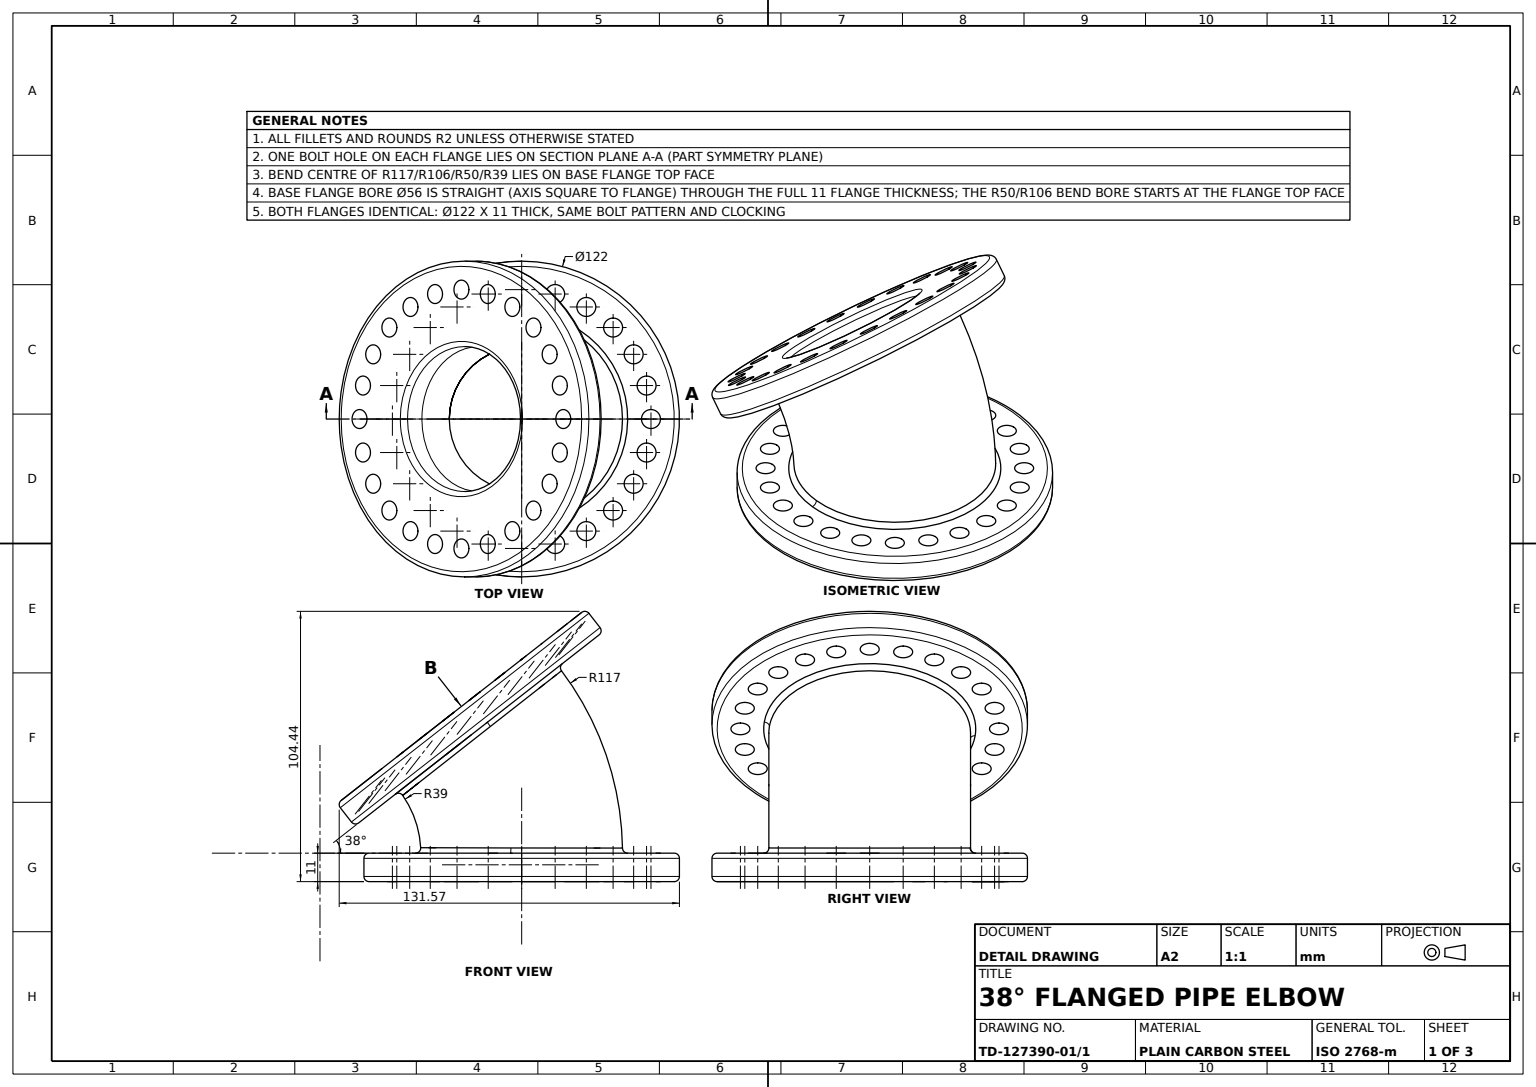
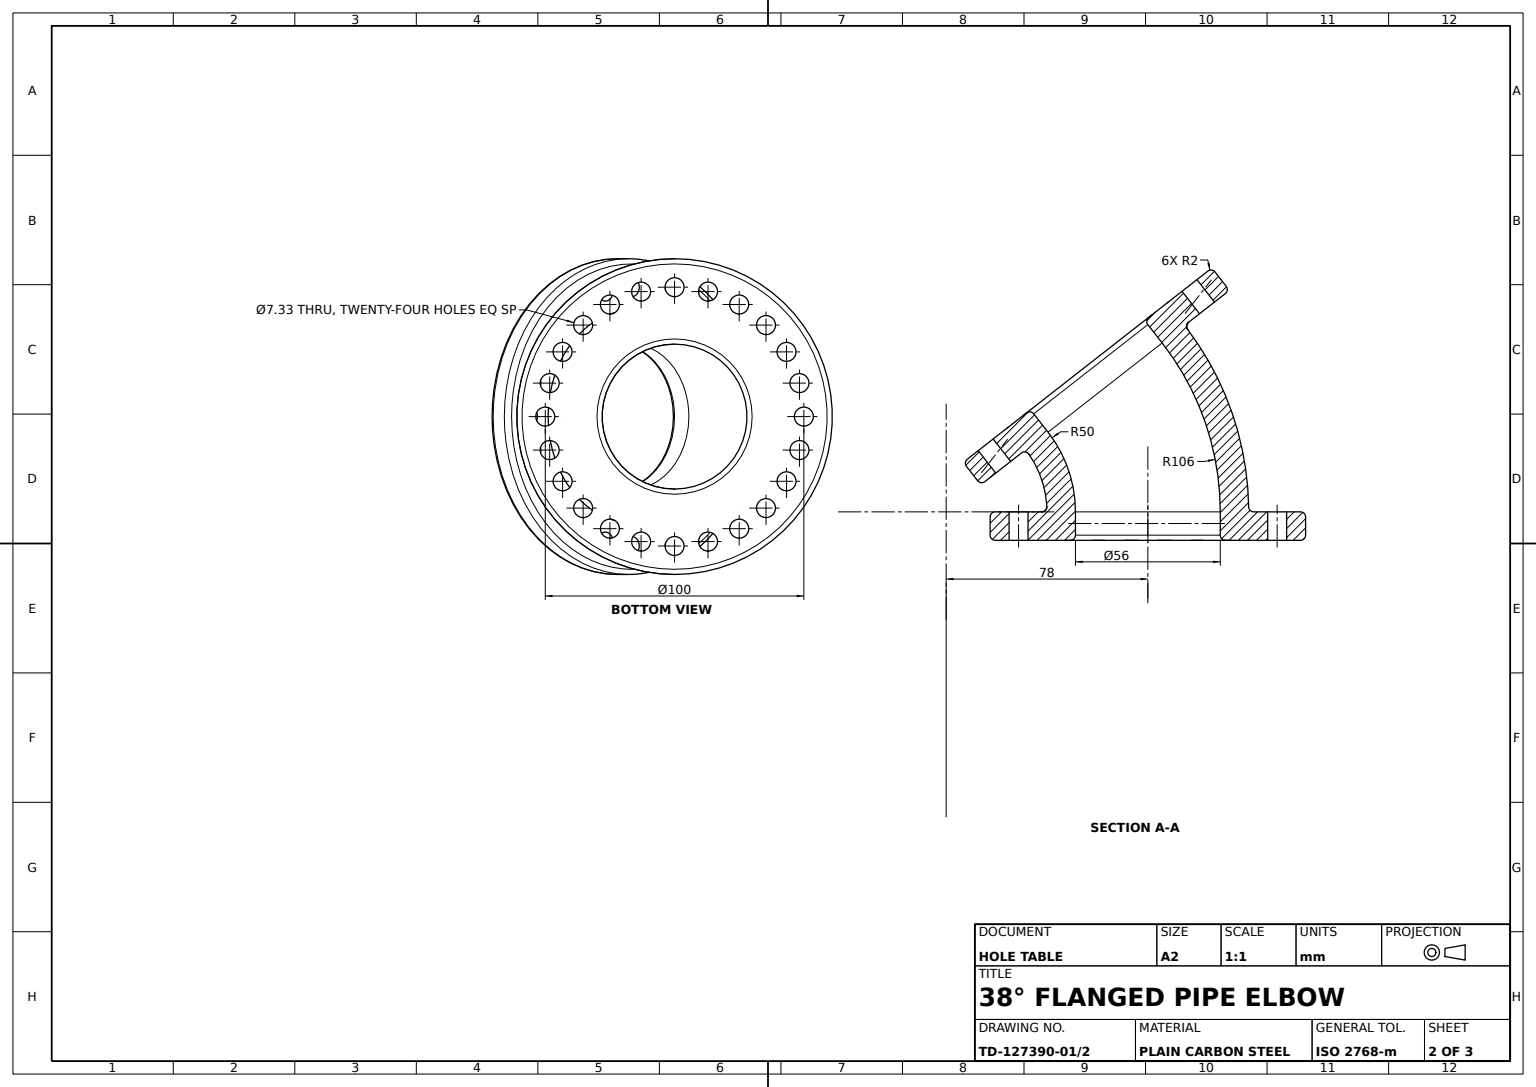
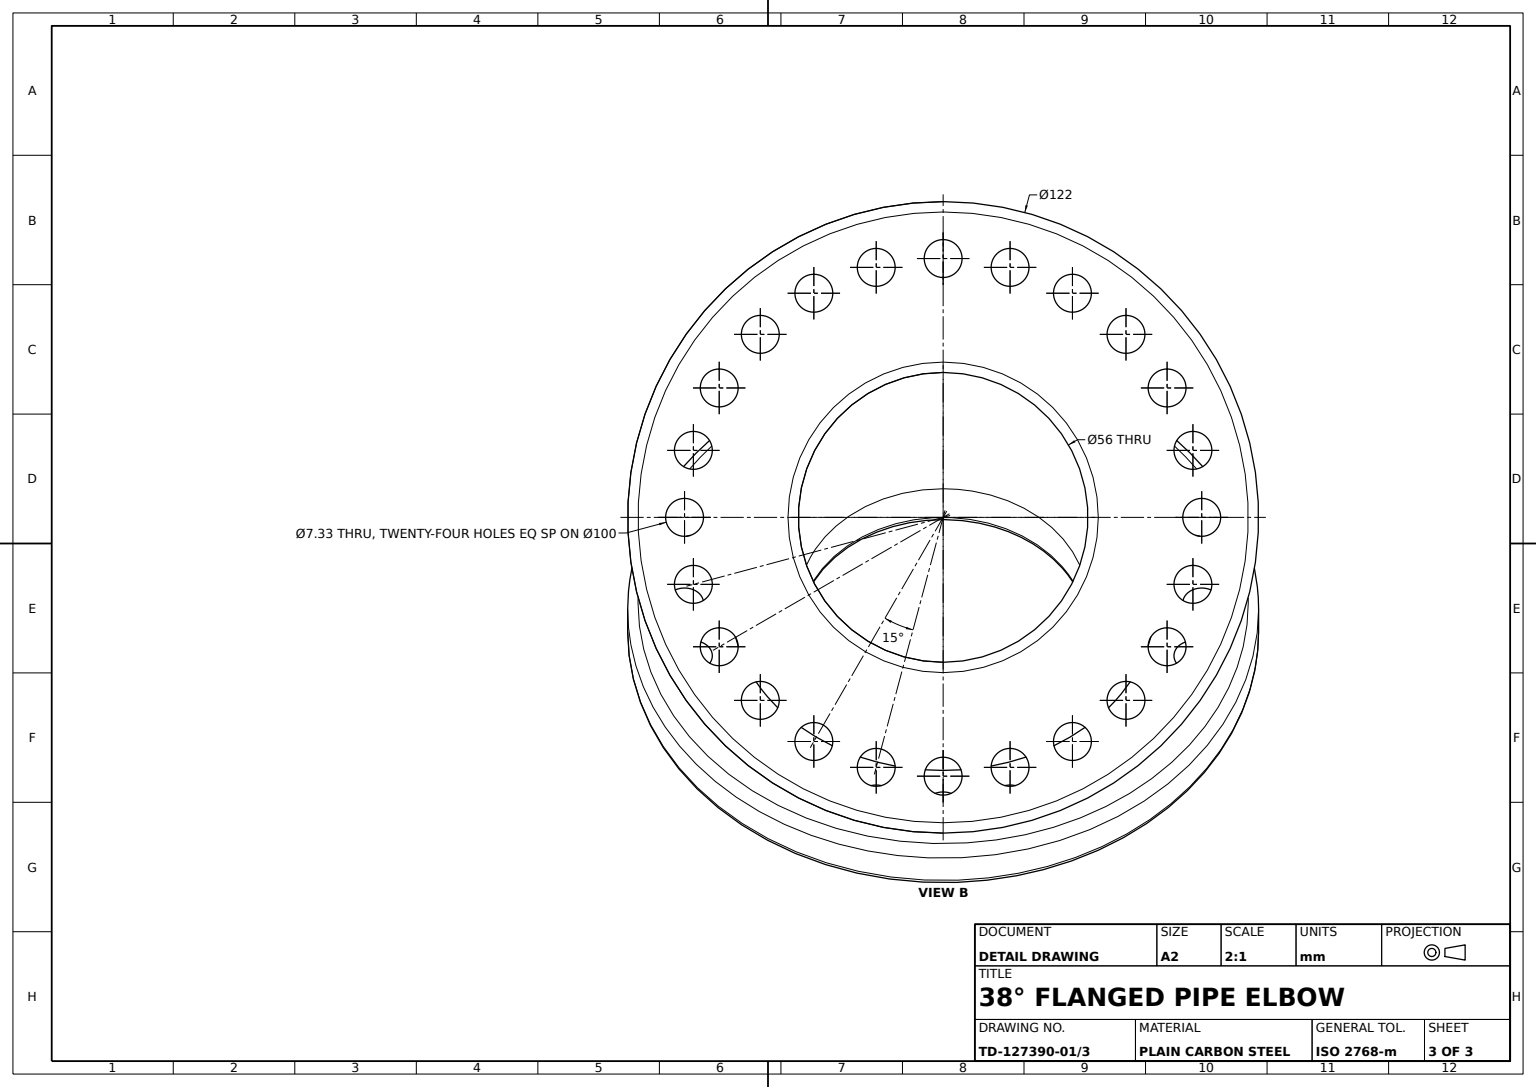
from build123d import *

# Parameters (mm, degrees)
BASE_FLANGE_SKETCH_R       = 61
BASE_FLANGE_SKETCH_R_2     = 28
BASE_FLANGE_SKETCH_R_3     = 3.665
BASE_FLANGE_24X_7_33_DEPTH = 11
BEND_PROFILE_SKETCH_R      = 39
BEND_PROFILE_SKETCH_R_2    = 28
PIPE_BEND_38DEG_ANGLE      = 38
END_FLANGE_SKETCH_R        = 61
END_FLANGE_SKETCH_R_2      = 28
END_FLANGE_SKETCH_R_3      = 3.665
END_FLANGE_24X_7_33_DEPTH  = 11
EDGE_FILLETS_R2_R          = 2


with BuildPart() as part:
    # Base Flange Sketch → Base Flange 24xØ7.33 (new body)
    with BuildSketch(Plane(origin=(0, 0, 0), x_dir=(1, 0, 0), z_dir=(0, 1, 0))):
        with Locations(Location((0, 0, 0), (0, 0, 270))):
            Circle(BASE_FLANGE_SKETCH_R)
        with Locations(Location((0, 0, 0), (0, 0, 270))):
            Circle(BASE_FLANGE_SKETCH_R_2, mode=Mode.SUBTRACT)
        with Locations(Location((0, 50, 0), (0, 0, 270))):
            Circle(BASE_FLANGE_SKETCH_R_3, mode=Mode.SUBTRACT)
        with Locations(Location((12.940952255, 48.296291314, 0), (0, 0, 270))):
            Circle(BASE_FLANGE_SKETCH_R_3, mode=Mode.SUBTRACT)
        with Locations(Location((25, 43.301270189, 0), (0, 0, 270))):
            Circle(BASE_FLANGE_SKETCH_R_3, mode=Mode.SUBTRACT)
        with Locations(Location((35.355339059, 35.355339059, 0), (0, 0, 270))):
            Circle(BASE_FLANGE_SKETCH_R_3, mode=Mode.SUBTRACT)
        with Locations(Location((43.301270189, 25, 0), (0, 0, 270))):
            Circle(BASE_FLANGE_SKETCH_R_3, mode=Mode.SUBTRACT)
        with Locations(Location((48.296291314, 12.940952255, 0), (0, 0, 270))):
            Circle(BASE_FLANGE_SKETCH_R_3, mode=Mode.SUBTRACT)
        with Locations(Location((50, 0, 0), (0, 0, 270))):
            Circle(BASE_FLANGE_SKETCH_R_3, mode=Mode.SUBTRACT)
        with Locations(Location((48.296291314, -12.940952255, 0), (0, 0, 270))):
            Circle(BASE_FLANGE_SKETCH_R_3, mode=Mode.SUBTRACT)
        with Locations(Location((43.301270189, -25, 0), (0, 0, 270))):
            Circle(BASE_FLANGE_SKETCH_R_3, mode=Mode.SUBTRACT)
        with Locations(Location((35.355339059, -35.355339059, 0), (0, 0, 270))):
            Circle(BASE_FLANGE_SKETCH_R_3, mode=Mode.SUBTRACT)
        with Locations(Location((25, -43.301270189, 0), (0, 0, 270))):
            Circle(BASE_FLANGE_SKETCH_R_3, mode=Mode.SUBTRACT)
        with Locations(Location((12.940952255, -48.296291314, 0), (0, 0, 270))):
            Circle(BASE_FLANGE_SKETCH_R_3, mode=Mode.SUBTRACT)
        with Locations(Location((0, -50, 0), (0, 0, 270))):
            Circle(BASE_FLANGE_SKETCH_R_3, mode=Mode.SUBTRACT)
        with Locations(Location((-12.940952255, -48.296291314, 0), (0, 0, 270))):
            Circle(BASE_FLANGE_SKETCH_R_3, mode=Mode.SUBTRACT)
        with Locations(Location((-25, -43.301270189, 0), (0, 0, 270))):
            Circle(BASE_FLANGE_SKETCH_R_3, mode=Mode.SUBTRACT)
        with Locations(Location((-35.355339059, -35.355339059, 0), (0, 0, 270))):
            Circle(BASE_FLANGE_SKETCH_R_3, mode=Mode.SUBTRACT)
        with Locations(Location((-43.301270189, -25, 0), (0, 0, 270))):
            Circle(BASE_FLANGE_SKETCH_R_3, mode=Mode.SUBTRACT)
        with Locations(Location((-48.296291314, -12.940952255, 0), (0, 0, 270))):
            Circle(BASE_FLANGE_SKETCH_R_3, mode=Mode.SUBTRACT)
        with Locations(Location((-50, 0, 0), (0, 0, 270))):
            Circle(BASE_FLANGE_SKETCH_R_3, mode=Mode.SUBTRACT)
        with Locations(Location((-48.296291314, 12.940952255, 0), (0, 0, 270))):
            Circle(BASE_FLANGE_SKETCH_R_3, mode=Mode.SUBTRACT)
        with Locations(Location((-43.301270189, 25, 0), (0, 0, 270))):
            Circle(BASE_FLANGE_SKETCH_R_3, mode=Mode.SUBTRACT)
        with Locations(Location((-35.355339059, 35.355339059, 0), (0, 0, 270))):
            Circle(BASE_FLANGE_SKETCH_R_3, mode=Mode.SUBTRACT)
        with Locations(Location((-25, 43.301270189, 0), (0, 0, 270))):
            Circle(BASE_FLANGE_SKETCH_R_3, mode=Mode.SUBTRACT)
        with Locations(Location((-12.940952255, 48.296291314, 0), (0, 0, 270))):
            Circle(BASE_FLANGE_SKETCH_R_3, mode=Mode.SUBTRACT)
    extrude(amount=-BASE_FLANGE_24X_7_33_DEPTH)

    # Bend Profile Sketch → Pipe Bend 38deg (revolve)
    with BuildSketch(Plane(origin=(0, 0, 0), x_dir=(1, 0, 0), z_dir=(0, 1, 0))):
        Circle(BEND_PROFILE_SKETCH_R)
        with Locations(Location((0, 0, 0), (0, 0, 270))):
            Circle(BEND_PROFILE_SKETCH_R_2, mode=Mode.SUBTRACT)
    revolve(axis=Axis((-78, 0, -90.684737963), (0, 0, 1)), revolution_arc=PIPE_BEND_38DEG_ANGLE)

    # End Flange Sketch → End Flange 24xØ7.33 (add)
    with BuildSketch(Plane(origin=(-29.565046072, 37.841533325, 0), x_dir=(0.7880107536067209, 0.6156614753256596, 0), z_dir=(-0.6156614753256596, 0.7880107536067209, 0))):
        with Locations(Location((16.535161219, 0, 0), (0, 0, 180))):
            Circle(END_FLANGE_SKETCH_R)
        with Locations((16.535161219, 0)):
            Circle(END_FLANGE_SKETCH_R_2, mode=Mode.SUBTRACT)
        with Locations(Location((16.535161219, 50, 0), (0, 0, 180))):
            Circle(END_FLANGE_SKETCH_R_3, mode=Mode.SUBTRACT)
        with Locations(Location((29.476113474, 48.296291314, 0), (0, 0, 180))):
            Circle(END_FLANGE_SKETCH_R_3, mode=Mode.SUBTRACT)
        with Locations(Location((41.535161219, 43.301270189, 0), (0, 0, 180))):
            Circle(END_FLANGE_SKETCH_R_3, mode=Mode.SUBTRACT)
        with Locations(Location((51.890500278, 35.355339059, 0), (0, 0, 180))):
            Circle(END_FLANGE_SKETCH_R_3, mode=Mode.SUBTRACT)
        with Locations(Location((59.836431408, 25, 0), (0, 0, 180))):
            Circle(END_FLANGE_SKETCH_R_3, mode=Mode.SUBTRACT)
        with Locations(Location((64.831452533, 12.940952255, 0), (0, 0, 180))):
            Circle(END_FLANGE_SKETCH_R_3, mode=Mode.SUBTRACT)
        with Locations(Location((66.535161219, 0, 0), (0, 0, 180))):
            Circle(END_FLANGE_SKETCH_R_3, mode=Mode.SUBTRACT)
        with Locations(Location((64.831452533, -12.940952255, 0), (0, 0, 180))):
            Circle(END_FLANGE_SKETCH_R_3, mode=Mode.SUBTRACT)
        with Locations(Location((59.836431408, -25, 0), (0, 0, 180))):
            Circle(END_FLANGE_SKETCH_R_3, mode=Mode.SUBTRACT)
        with Locations(Location((51.890500278, -35.355339059, 0), (0, 0, 180))):
            Circle(END_FLANGE_SKETCH_R_3, mode=Mode.SUBTRACT)
        with Locations(Location((41.535161219, -43.301270189, 0), (0, 0, 180))):
            Circle(END_FLANGE_SKETCH_R_3, mode=Mode.SUBTRACT)
        with Locations(Location((29.476113474, -48.296291314, 0), (0, 0, 180))):
            Circle(END_FLANGE_SKETCH_R_3, mode=Mode.SUBTRACT)
        with Locations(Location((16.535161219, -50, 0), (0, 0, 180))):
            Circle(END_FLANGE_SKETCH_R_3, mode=Mode.SUBTRACT)
        with Locations(Location((3.594208964, -48.296291314, 0), (0, 0, 180))):
            Circle(END_FLANGE_SKETCH_R_3, mode=Mode.SUBTRACT)
        with Locations(Location((-8.464838781, -43.301270189, 0), (0, 0, 180))):
            Circle(END_FLANGE_SKETCH_R_3, mode=Mode.SUBTRACT)
        with Locations(Location((-18.820177841, -35.355339059, 0), (0, 0, 180))):
            Circle(END_FLANGE_SKETCH_R_3, mode=Mode.SUBTRACT)
        with Locations(Location((-26.766108971, -25, 0), (0, 0, 180))):
            Circle(END_FLANGE_SKETCH_R_3, mode=Mode.SUBTRACT)
        with Locations(Location((-31.761130096, -12.940952255, 0), (0, 0, 180))):
            Circle(END_FLANGE_SKETCH_R_3, mode=Mode.SUBTRACT)
        with Locations(Location((-33.464838781, 0, 0), (0, 0, 180))):
            Circle(END_FLANGE_SKETCH_R_3, mode=Mode.SUBTRACT)
        with Locations(Location((-31.761130096, 12.940952255, 0), (0, 0, 180))):
            Circle(END_FLANGE_SKETCH_R_3, mode=Mode.SUBTRACT)
        with Locations(Location((-26.766108971, 25, 0), (0, 0, 180))):
            Circle(END_FLANGE_SKETCH_R_3, mode=Mode.SUBTRACT)
        with Locations(Location((-18.820177841, 35.355339059, 0), (0, 0, 180))):
            Circle(END_FLANGE_SKETCH_R_3, mode=Mode.SUBTRACT)
        with Locations(Location((-8.464838781, 43.301270189, 0), (0, 0, 180))):
            Circle(END_FLANGE_SKETCH_R_3, mode=Mode.SUBTRACT)
        with Locations(Location((3.594208964, 48.296291314, 0), (0, 0, 180))):
            Circle(END_FLANGE_SKETCH_R_3, mode=Mode.SUBTRACT)
    extrude(amount=END_FLANGE_24X_7_33_DEPTH)

    # Edge Fillets R2
    edge_fillets_r2_edges = [part.edges().sort_by_distance(p)[0] for p in [
        (-39, 0, 0),
        (-47.267580609, 24.010797538, 0),
        (24.761218523, 94.24506336, 0),
        (31.533494751, 85.57694507, 0),
        (-45.371738548, 39.451192056, 0),
        (0, 0, -61),
        (0, -11, -61),
        (0, -11, -28),
    ]]
    fillet(edge_fillets_r2_edges, radius=EDGE_FILLETS_R2_R)


solid = part.part
